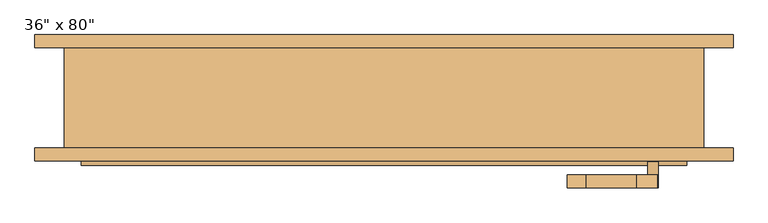
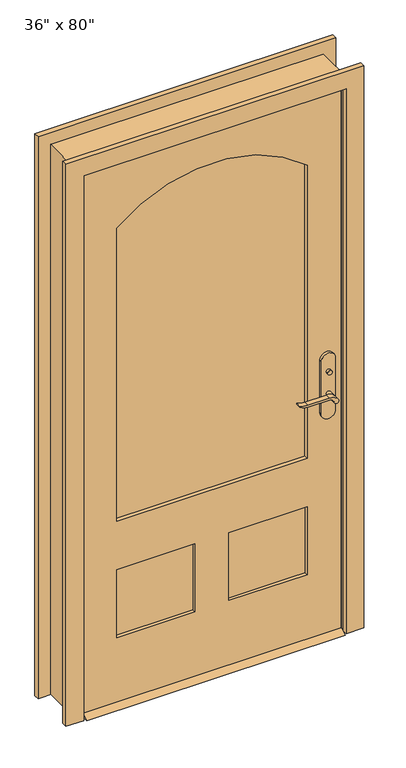
"""IFC4 building model written with IfcOpenShell, lengths in millimetres: door geometry."""

from ifc_helpers import new_model, si_unit, point, frame, frame_2d, origin, place, context, project, spatial, polyline, circle_curve, trimmed, segment, composite_curve, outline, extrude, faceted_brep, source, transform, mapped, element, save


def door_5d363d20(model_context):
    return source(origin(), model_context, "Body", "SolidModel", [
        extrude(outline(polyline([(-38.1, 12.7), (-12.7, 0.0), (-98.425, 0.0), (-73.025, 12.7), (-38.1, 12.7)])), frame((-457.2, 0.0, 0.0), z_axis=(1.0, 0.0, 0.0), x_axis=(0.0, 1.0, 0.0)), (0.0, 0.0, 1.0), 914.4),
        extrude(outline(polyline([(411.4, -18.1), (411.4, -28.1), (401.4, -28.1), (401.4, -18.1), (411.4, -18.1)])), frame((0.0, 0.0, 981.9), z_axis=(0.0, 0.0, 1.0), x_axis=(1.0, 0.0, 0.0)), (0.0, 0.0, 1.0), 30.0),
        extrude(outline(composite_curve([segment(trimmed(circle_curve(frame_2d((996.9, 406.4)), 8.0), [point((996.9, 398.4))], [point((996.9, 414.4))], False, "CARTESIAN"), True, "CONTINUOUS"), segment(trimmed(circle_curve(frame_2d((996.9, 406.4)), 8.0), [point((996.9, 414.4))], [point((996.9, 398.4))], False, "CARTESIAN"), True, "CONTINUOUS")], self_intersect=False)), frame((0.0, -93.025, 0.0), z_axis=(0.0, 1.0, 0.0), x_axis=(0.0, 0.0, 1.0)), (0.0, 0.0, 1.0), 10.0),
        extrude(outline(composite_curve([segment(trimmed(circle_curve(frame_2d((897.1555521, 382.7324871)), 37.2832219), [point((919.0523287, 412.9081363))], [point((934.4, 381.0325667))], False, "CARTESIAN"), True, "CONTINUOUS"), segment(polyline([(934.4, 381.0325667), (934.4, 304.7564091)]), True, "CONTINUOUS"), segment(trimmed(circle_curve(frame_2d((1017.6850638, 304.8227909)), 83.2850902), [point((934.4, 304.7564091))], [point((939.4, 276.4))], True, "CARTESIAN"), True, "CONTINUOUS"), segment(polyline([(939.4, 276.4), (936.6135558, 276.4)]), True, "CONTINUOUS"), segment(trimmed(circle_curve(frame_2d((986.6709207, 308.3396612)), 59.3791355), [point((936.6135558, 276.4))], [point((927.4, 304.7564091))], False, "CARTESIAN"), True, "CONTINUOUS"), segment(polyline([(927.4, 304.7564091), (927.4, 381.0138099)]), True, "CONTINUOUS"), segment(trimmed(circle_curve(frame_2d((909.2738613, 381.0138099)), 18.1261387), [point((927.4, 381.0138099))], [point((914.4, 398.4))], True, "CARTESIAN"), True, "CONTINUOUS"), segment(trimmed(circle_curve(frame_2d((914.4, 406.4)), 8.0), [point((914.4, 398.4))], [point((919.0523287, 412.9081363))], False, "CARTESIAN"), True, "CONTINUOUS")], self_intersect=False)), frame((0.0, 1.9, 0.0), z_axis=(0.0, 1.0, 0.0), x_axis=(0.0, 0.0, 1.0)), (0.0, 0.0, 1.0), 20.0),
        extrude(outline(composite_curve([segment(trimmed(circle_curve(frame_2d((914.4, 406.4)), 8.0), [point((914.3999903, 398.4))], [point((919.0523287, 412.9081363))], False, "CARTESIAN"), True, "CONTINUOUS"), segment(trimmed(circle_curve(frame_2d((897.1555521, 382.7324871)), 37.2832219), [point((919.0523287, 412.9081363))], [point((934.4, 381.0325667))], False, "CARTESIAN"), True, "CONTINUOUS"), segment(polyline([(934.4, 381.0325667), (934.4, 304.7564091)]), True, "CONTINUOUS"), segment(trimmed(circle_curve(frame_2d((1017.6850638, 304.8227909)), 83.2850902), [point((934.4, 304.7564091))], [point((939.4, 276.4))], True, "CARTESIAN"), True, "CONTINUOUS"), segment(polyline([(939.4, 276.4), (936.6135558, 276.4)]), True, "CONTINUOUS"), segment(trimmed(circle_curve(frame_2d((986.6709207, 308.3396612)), 59.3791355), [point((936.6135558, 276.4))], [point((927.4, 304.7564091))], False, "CARTESIAN"), True, "CONTINUOUS"), segment(polyline([(927.4, 304.7564091), (927.4, 381.0138122)]), True, "CONTINUOUS"), segment(trimmed(circle_curve(frame_2d((909.2738682, 381.0138122)), 18.1261318), [point((927.4, 381.0138122))], [point((914.3999903, 398.4))], True, "CARTESIAN"), True, "CONTINUOUS")], self_intersect=False)), frame((0.0, -133.025, 0.0), z_axis=(0.0, 1.0, 0.0), x_axis=(0.0, 0.0, 1.0)), (0.0, 0.0, 1.0), 20.0),
        extrude(outline(composite_curve([segment(trimmed(circle_curve(frame_2d((914.4, 406.4)), 8.0), [point((914.4, 398.4))], [point((914.4, 414.4))], False, "CARTESIAN"), True, "CONTINUOUS"), segment(trimmed(circle_curve(frame_2d((914.4, 406.4)), 8.0), [point((914.4, 414.4))], [point((914.4, 398.4))], False, "CARTESIAN"), True, "CONTINUOUS")], self_intersect=False)), frame((0.0, -28.1, 0.0), z_axis=(0.0, 1.0, 0.0), x_axis=(0.0, 0.0, 1.0)), (0.0, 0.0, 1.0), 30.0),
        extrude(outline(composite_curve([segment(trimmed(circle_curve(frame_2d((914.4, 406.4)), 8.0), [point((914.4, 398.4))], [point((914.4, 414.4))], False, "CARTESIAN"), True, "CONTINUOUS"), segment(trimmed(circle_curve(frame_2d((914.4, 406.4)), 8.0), [point((914.4, 414.4))], [point((914.4, 398.4))], False, "CARTESIAN"), True, "CONTINUOUS")], self_intersect=False)), frame((0.0, -113.025, 0.0), z_axis=(0.0, 1.0, 0.0), x_axis=(0.0, 0.0, 1.0)), (0.0, 0.0, 1.0), 30.0),
        extrude(outline(composite_curve([segment(polyline([(844.4, 431.4), (1039.4, 431.4)]), True, "CONTINUOUS"), segment(trimmed(circle_curve(frame_2d((1039.4, 406.4)), 25.0), [point((1039.4, 431.4))], [point((1039.4, 381.4))], False, "CARTESIAN"), True, "CONTINUOUS"), segment(polyline([(1039.4, 381.4), (844.4, 381.4)]), True, "CONTINUOUS"), segment(trimmed(circle_curve(frame_2d((844.4, 406.4)), 25.0), [point((844.4, 381.4))], [point((844.4, 431.4))], False, "CARTESIAN"), True, "CONTINUOUS")], self_intersect=False)), frame((0.0, -38.1, 0.0), z_axis=(0.0, 1.0, 0.0), x_axis=(0.0, 0.0, 1.0)), (0.0, 0.0, 1.0), 10.0),
        extrude(outline(composite_curve([segment(polyline([(844.4, 431.4), (1039.4, 431.4)]), True, "CONTINUOUS"), segment(trimmed(circle_curve(frame_2d((1039.4, 406.4)), 25.0), [point((1039.4, 431.4))], [point((1039.4, 381.4))], False, "CARTESIAN"), True, "CONTINUOUS"), segment(polyline([(1039.4, 381.4), (844.4, 381.4)]), True, "CONTINUOUS"), segment(trimmed(circle_curve(frame_2d((844.4, 406.4)), 25.0), [point((844.4, 381.4))], [point((844.4, 431.4))], False, "CARTESIAN"), True, "CONTINUOUS")], self_intersect=False)), frame((0.0, -83.025, 0.0), z_axis=(0.0, 1.0, 0.0), x_axis=(0.0, 0.0, 1.0)), (0.0, 0.0, 1.0), 10.0),
        extrude(outline(polyline([(2032.0, -457.2), (12.7, -457.2), (12.7, 457.2), (2032.0, 457.2), (2032.0, -457.2)]), holes=[composite_curve([segment(polyline([(688.975, -336.55), (1784.35, -336.55)]), True, "CONTINUOUS"), segment(trimmed(circle_curve(frame_2d((1401.92125, 0.0)), 509.42875), [point((1784.35, -336.55))], [point((1784.35, 336.55))], True, "CARTESIAN"), True, "CONTINUOUS"), segment(polyline([(1784.35, 336.55), (688.975, 336.55), (688.975, -336.55)]), True, "CONTINUOUS")], self_intersect=False), polyline([(508.0, -60.325), (254.0, -60.325), (254.0, -336.55), (508.0, -336.55), (508.0, -60.325)]), polyline([(508.0, 336.55), (254.0, 336.55), (254.0, 60.325), (508.0, 60.325), (508.0, 336.55)])]), frame((0.0, -73.025, 0.0), z_axis=(0.0, 1.0, 0.0), x_axis=(0.0, 0.0, 1.0)), (0.0, 0.0, 1.0), 34.925),
        faceted_brep([(482.6, -73.025, 0.0), (457.2, -73.025, 0.0), (457.2, -38.1, 0.0), (444.5, -38.1, 0.0), (444.5, -3.175, 0.0), (457.2, -3.175, 0.0), (457.2, 79.375, 0.0), (482.6, 79.375, 0.0), (482.6, 79.375, 2057.4), (482.6, -73.025, 2057.4), (457.2, 79.375, 2032.0), (-457.2, 79.375, 2032.0), (-457.2, 79.375, 0.0), (-482.6, 79.375, 0.0), (-482.6, 79.375, 2057.4), (457.2, -3.175, 2032.0), (444.5, -3.175, 2019.3), (-444.5, -3.175, 2019.3), (-444.5, -3.175, 0.0), (-457.2, -3.175, 0.0), (-457.2, -3.175, 2032.0), (444.5, -38.1, 2019.3), (457.2, -38.1, 2032.0), (-457.2, -38.1, 2032.0), (-457.2, -38.1, 0.0), (-444.5, -38.1, 0.0), (-444.5, -38.1, 2019.3), (457.2, -73.025, 2032.0), (-482.6, -73.025, 2057.4), (-482.6, -73.025, 0.0), (-457.2, -73.025, 0.0), (-457.2, -73.025, 2032.0)], [[[0, 1, 2, 3, 4, 5, 6, 7]], [[7, 8, 9, 0]], [[6, 10, 11, 12, 13, 14, 8, 7]], [[5, 15, 10, 6]], [[4, 16, 17, 18, 19, 20, 15, 5]], [[3, 21, 16, 4]], [[2, 22, 23, 24, 25, 26, 21, 3]], [[1, 27, 22, 2]], [[0, 9, 28, 29, 30, 31, 27, 1]], [[8, 14, 28, 9]], [[15, 20, 11, 10]], [[21, 26, 17, 16]], [[27, 31, 23, 22]], [[29, 13, 12, 19, 18, 25, 24, 30]], [[14, 13, 29, 28]], [[20, 19, 12, 11]], [[26, 25, 18, 17]], [[31, 30, 24, 23]]]),
        extrude(outline(polyline([(-60.325, -49.7416667), (-60.325, -61.3833333), (-336.55, -61.3833333), (-336.55, -49.7416667), (-60.325, -49.7416667)])), frame((0.0, 0.0, 254.0), z_axis=(0.0, 0.0, 1.0), x_axis=(1.0, 0.0, 0.0)), (0.0, 0.0, 1.0), 254.0),
        extrude(outline(polyline([(336.55, -49.7416667), (336.55, -61.3833333), (60.325, -61.3833333), (60.325, -49.7416667), (336.55, -49.7416667)])), frame((0.0, 0.0, 254.0), z_axis=(0.0, 0.0, 1.0), x_axis=(1.0, 0.0, 0.0)), (0.0, 0.0, 1.0), 254.0),
        extrude(outline(composite_curve([segment(polyline([(688.975, -336.55), (688.975, 336.55), (1784.35, 336.55)]), True, "CONTINUOUS"), segment(trimmed(circle_curve(frame_2d((1401.92125, 0.0)), 509.42875), [point((1784.35, 336.55))], [point((1784.35, -336.55))], False, "CARTESIAN"), True, "CONTINUOUS"), segment(polyline([(1784.35, -336.55), (688.975, -336.55)]), True, "CONTINUOUS")], self_intersect=False)), frame((0.0, -59.055, 0.0), z_axis=(0.0, 1.0, 0.0), x_axis=(0.0, 0.0, 1.0)), (0.0, 0.0, 1.0), 6.985),
        extrude(outline(polyline([(0.0, -463.55), (2038.35, -463.55), (2038.35, 463.55), (0.0, 463.55), (0.0, 527.05), (2101.85, 527.05), (2101.85, -527.05), (0.0, -527.05), (0.0, -463.55)])), frame((0.0, 79.375, 0.0), z_axis=(0.0, 1.0, 0.0), x_axis=(0.0, 0.0, 1.0)), (0.0, 0.0, 1.0), 19.05),
        extrude(outline(polyline([(0.0, -463.55), (2038.35, -463.55), (2038.35, 463.55), (0.0, 463.55), (0.0, 527.05), (2101.85, 527.05), (2101.85, -527.05), (0.0, -527.05), (0.0, -463.55)])), frame((0.0, -92.075, 0.0), z_axis=(0.0, 1.0, 0.0), x_axis=(0.0, 0.0, 1.0)), (0.0, 0.0, 1.0), 19.05),
    ])


if __name__ == "__main__":
    model = new_model("IFC4")
    model_context = context("Model", 3, world=origin())
    ifc_project = project(units=[si_unit("LENGTHUNIT", "METRE", prefix="MILLI")], contexts=[model_context])
    site = spatial("IfcSite", under=ifc_project)
    building = spatial("IfcBuilding", under=site)
    placement = place(None, origin())
    door_shape = door_5d363d20(model_context)
    element("IfcDoor", 1, ObjectType="36\" x 80\"", at=placement, inside=building, context=model_context, shape_type="MappedRepresentation", body=[
        mapped(door_shape, transform((0.0, 0.0, 0.0), x_axis=(1.0, 0.0, 0.0), y_axis=(0.0, 1.0, 0.0), z_axis=(0.0, 0.0, 1.0))),
    ])
    save(model, "model.ifc")

# Revit data of these elements
# Type "36\" x 80\""
#   Type Mark = "9"
#   Assembly Code = "B2030100"
#   Analytic Construction = "French door, wood frame with single glass"
#   Threshold Offset [instance default] = 0' - 0 1/2"
#   Thickness = 0' - 1 3/8"
#   Thermal Resistance (R) = 1.0696 (h·ft²·°F)/BTU
#   Swing Angle [instance default] = 90.00°
#   Stiles = 0' - 4 3/4"
#   Rough Width = 3' - 2"
#   Rough Height = 6' - 9"
#   Radius = 1' - 8.05625"
#   Lock Rail = 0' - 7 1/8"
#   Height = 6' - 8"
#   Width = 3' - 0"
#   Heat Transfer Coefficient (U) = 0.9350 BTU/(h·ft²·°F)
#   Door Offset [instance default] = 0' - 0"
#   Bottom Rail = 0' - 9 1/2"
#   Threshold [instance default] = yes
#   Function = 1
#   Exterior Trim [instance default] = yes
#   Trim Material = Cherry
#   Threshold Material = Cherry
#   Panel Material = Cherry
#   Glazing = Glass
#   Frame Material = Cherry
#   Door Handle Material = Aluminum
#   Visual Light Transmittance = 0
#   Solar Heat Gain Coefficient = 0
#   Wall Closure = (empty or 0)
#   Construction Type = (empty or 0)
# Element 1 (IfcDoor, "36\" x 80\"")
#   Materials on its faces: "Cherry", "Aluminum", "Glass"
# Materials
#   "Cherry": class "Wood", colour RGB 226 177 128, transparency 0, Description = "Prunus Serotina", Cost = 0
#   "Glass": class "Glass", colour RGB 0 128 192, transparency 0.75, Description = "Soda Lime Glass", Cost = 0
#   "Aluminum": class "Metal", colour RGB 247 247 247, transparency 0, Description = "Aluminum 6061", Cost = 0
